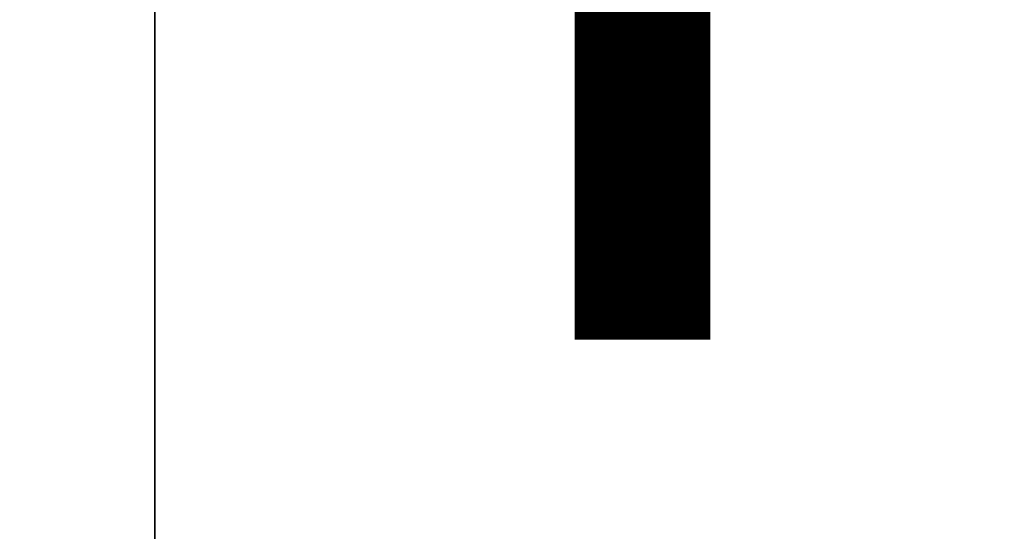
# Model space of a CAD drawing. Units: inches. Extents: x 2083 to 3317, y 1141 to 2115.
# Tile 23 of 256: x 2225.819 to 2234.135, y 1481.434 to 1485.751. Entities that reach past the tile are written whole.
import ezdxf

# ---------------------------------------------------------------- set-up
doc = ezdxf.new("R2010")
doc.units = ezdxf.units.IN
doc.layers.add('A-ANNO-DIMS', color=2, linetype='Continuous', lineweight=18)
doc.layers.add('A-WALL', color=7, linetype='Continuous', lineweight=35)
doc.layers.add('A-WALL-PATT', color=251, linetype='Continuous', lineweight=13, true_color=0x636466)
doc.styles.get("Standard").update_dxf_attribs({"font": 'arial.ttf'})
doc.dimstyles.new('ISO-25', dxfattribs={"dimtxt": 12, "dimasz": 12, "dimexe": 1.25, "dimexo": 0.625, "dimtad": 1, "dimlunit": 3, "dimtxsty": 'Standard', "dimcen": 2.5, "dimadec": 0, "dimazin": 0, "dimtfac": 1, "dimtmove": 0, "dimatfit": 3, "dimfxl": 1, "dimarcsym": 0})

# ---------------------------------------------------------------- blocks, each defined once
blk = doc.blocks.new('*D30')
at = {"layer": 'A-ANNO-DIMS', "color": 0, "lineweight": -2, "transparency": 16777216}
for p, q in [((2240.0179, 1445.2738), (2240.0179, 1448.0455)), ((2254.3293, 1445.2738), (2254.3293, 1448.0455)), ((2228.0179, 1446.7955), (2216.0179, 1446.7955)), ((2240.0179, 1446.7955), (2254.3293, 1446.7955)), ((2266.3293, 1446.7955), (2413.7649, 1446.7955))]:
    blk.add_line(p, q, dxfattribs=at)
at = {"layer": 'A-ANNO-DIMS', "color": 0, "transparency": 16777216}
for points in [[(2228.0179, 1448.7955), (2228.0179, 1444.7955), (2240.0179, 1446.7955)], [(2266.3293, 1448.7955), (2266.3293, 1444.7955), (2254.3293, 1446.7955)]]:
    blk.add_solid(points, dxfattribs=at)
at = {"layer": 'Defpoints', "color": 0, "transparency": 16777216}
for p in [(2254.3293, 1446.7955), (2240.0179, 1444.6488), (2254.3293, 1444.6488)]:
    blk.add_point(p, dxfattribs=at)
at = {"layer": 'A-ANNO-DIMS', "color": 0, "transparency": 16777216, "insert": (2346.0471, 1453.6252), "char_height": 12, "attachment_point": 5}
blk.add_mtext('WC 1\'-2 1/2" TYP.', dxfattribs=at)
blk = doc.blocks.new('*D31')
at = {"layer": 'A-ANNO-DIMS', "color": 0, "lineweight": -2, "transparency": 16777216}
for p, q in [((2237.8711, 1456.6488), (2237.8711, 1541.9152)), ((2239.3929, 1444.6488), (2236.6211, 1444.6488)), ((2237.8711, 1431.5475), (2237.8711, 1444.6488)), ((2239.3929, 1431.5475), (2236.6211, 1431.5475)), ((2237.8711, 1419.5475), (2237.8711, 1407.5475))]:
    blk.add_line(p, q, dxfattribs=at)
at = {"layer": 'A-ANNO-DIMS', "color": 0, "transparency": 16777216}
for points in [[(2235.8711, 1456.6488), (2239.8711, 1456.6488), (2237.8711, 1444.6488)], [(2235.8711, 1419.5475), (2239.8711, 1419.5475), (2237.8711, 1431.5475)]]:
    blk.add_solid(points, dxfattribs=at)
at = {"layer": 'Defpoints', "color": 0, "transparency": 16777216}
for p in [(2237.8711, 1444.6488), (2240.0179, 1444.6488), (2240.0179, 1431.5475)]:
    blk.add_point(p, dxfattribs=at)
at = {"layer": 'A-ANNO-DIMS', "color": 0, "transparency": 16777216, "insert": (2231.2175, 1505.282), "char_height": 12, "attachment_point": 5, "rotation": 90}
blk.add_mtext('1\'-1" TYP.', dxfattribs=at)

msp = doc.modelspace()

# ---------------------------------------------------------------- hatches: boundary and pattern name
at = {"layer": 'A-WALL-PATT'}
h = msp.add_hatch(color=256, dxfattribs=at)
h.dxf.hatch_style = 1
h.paths.add_polyline_path([(3126.9598, 2020.7614), (2748.9598, 2020.7614), (2604.9598, 2020.7614), (2226.9598, 2020.7614), (2226.9598, 1702.7614), (2466.9598, 1702.7614), (2466.9598, 1582.7614), (2418.9598, 1582.7614), (2418.9598, 1477.7614), (2226.9598, 1477.7614), (2226.9598, 1263.2614), (2544.9598, 1263.2614), (2544.9598, 1411.7614), (2604.9598, 1411.7614), (2685.9598, 1411.7614), (2685.9598, 1420.7614), (2604.9598, 1420.7614), (2604.9598, 1573.7614), (2604.9598, 1702.7614), (2604.9598, 2011.7614), (2748.9598, 2011.7614), (2748.9598, 1702.7614), (2862.9598, 1702.7614), (2862.9598, 1621.7614), (2871.9598, 1621.7614), (2871.9598, 1702.7614), (2883.9598, 1702.7614), (2883.9598, 1706.9395, -0.026459), (2883.9598, 1711.7614), (2757.9598, 1711.7614), (2757.9598, 1807.7614), (2787.9598, 1807.7614), (2787.9598, 1812.2614), (2757.9598, 1812.2614), (2757.9598, 2011.7614), (2877.9598, 2011.7614), (2877.9598, 1812.2614), (2847.9598, 1812.2614), (2847.9598, 1807.7614), (2889.8357, 1807.7614), (2889.8357, 1812.2614), (2882.4598, 1812.2614), (2882.4598, 2011.7614), (3117.9598, 2011.7614), (3117.9598, 1812.2614), (2937.8357, 1812.2614), (2937.8357, 1807.7614), (2995.7098, 1807.7614), (2995.7098, 1796.1177), (3000.2098, 1796.1177), (3000.2098, 1807.7614), (3117.9598, 1807.7614), (3117.9598, 1711.7614), (3000.2098, 1711.7614), (3000.2098, 1760.1177), (2998.5727, 1760.1177, -0.020711), (2995.7098, 1760.1177), (2995.7098, 1711.7614), (2931.9598, 1711.7614), (2931.9598, 1702.7614), (3126.9598, 1702.7614)])
h.paths.add_polyline_path([(2471.4598, 2011.7614), (2471.4598, 1810.0114), (2462.7169, 1810.0114), (2462.7169, 1805.5114), (2505.9598, 1805.5114), (2505.9598, 1810.0114), (2475.9598, 1810.0114), (2475.9598, 2011.7614), (2595.9598, 2011.7614), (2595.9598, 1810.0114), (2565.9598, 1810.0114), (2565.9598, 1805.5114), (2595.9598, 1805.5114), (2595.9598, 1711.7614), (2235.9598, 1711.7614), (2235.9598, 1805.5114), (2353.7098, 1805.5114), (2353.7098, 1796.0542), (2358.2098, 1796.0542), (2358.2098, 1805.5114), (2414.7169, 1805.5114), (2414.7169, 1810.0114), (2235.9598, 1810.0114), (2235.9598, 2011.7614)], flags=16)
h.paths.add_polyline_path([(2270.2047, 1994.61), (2270.2047, 1970.61), (2246.2047, 1970.61), (2246.2047, 1994.61)], flags=0)
edge = h.paths.add_edge_path(flags=0)
edge.add_ellipse((2332.0274, 1899.7982), major_axis=(-3.043, 3.043), ratio=0.168252, start_angle=-161.33217, end_angle=-156.30711, ccw=False)
edge.add_ellipse((2333.082, 1898.7435), major_axis=(-1.0546, 1.0546), ratio=0.453532, start_angle=-123.37102, end_angle=-94.15911)
edge = h.paths.add_edge_path(flags=0)
edge.add_ellipse((2332.0274, 1968.8763), major_axis=(3.043, 3.043), ratio=0.168252, start_angle=18.66783, end_angle=23.69289)
edge.add_spline(control_points=[(2332.9256, 1970.6911), (2332.2268, 1970.3361), (2330.8937, 1969.6589), (2328.4131, 1970.9321), (2327.2039, 1967.7487), (2324.7096, 1969.9556), (2322.5328, 1967.0124), (2320.0128, 1971.2958), (2317.6803, 1968.1578), (2316.0405, 1967.102), (2315.4269, 1966.8096)], knot_values=[0, 0, 0, 0, 2.267059, 4.324559, 6.685584, 8.878641, 11.121502, 14.300359, 17.755284, 19.732645, 19.732645, 19.732645, 19.732645], degree=3, periodic=0)
edge.add_ellipse((2332.0274, 1968.8763), major_axis=(3.043, 3.043), ratio=0.168252, start_angle=18.66783, end_angle=23.69289, ccw=False)
edge.add_ellipse((2333.082, 1969.9309), major_axis=(1.0546, 1.0546), ratio=0.453532, start_angle=56.62898, end_angle=85.84089, ccw=False)
edge = h.paths.add_edge_path(flags=0)
edge.add_spline(control_points=[(2296.4283, 1967.9879), (2293.6278, 1965.3363), (2287.7036, 1959.7271), (2299.7439, 1949.9957), (2294.5326, 1935.6685), (2290.5732, 1920.6035), (2293.3941, 1909.9737), (2296.1854, 1904.9665)], knot_values=[0.099185, 0.099185, 0.099185, 0.099185, 0.345301, 0.619822, 0.982653, 1.386093, 1.810555, 1.810555, 1.810555, 1.810555], degree=3, periodic=0)
edge.add_spline(control_points=[(2296.1854, 1904.9665), (2297.3836, 1902.6193), (2298.001, 1901.9493), (2298.553, 1901.4682)], knot_values=[0.006246, 0.006246, 0.006246, 0.006246, 0.055476, 0.055476, 0.055476, 0.055476], degree=3, periodic=0)
edge.add_spline(control_points=[(2298.553, 1901.4682), (2297.2586, 1900.9232), (2295.2253, 1900.2321), (2293.0602, 1900.6142), (2292.1014, 1900.7884), (2292.0896, 1900.7906)], knot_values=[0.312835, 0.312835, 0.312835, 0.312835, 0.40178, 0.474987, 0.475903, 0.475903, 0.475903, 0.475903], degree=3, periodic=0)
edge.add_arc((2292.7936, 1904.6641), 3.937, 215.4209, 259.69818, ccw=False)
edge.add_spline(control_points=[(2289.5853, 1902.3823), (2289.4767, 1902.5351), (2289.3685, 1902.688), (2289.2609, 1902.8412)], knot_values=[0.102872, 0.102872, 0.102872, 0.102872, 0.116896, 0.116896, 0.116896, 0.116896], degree=3, periodic=0)
edge.add_spline(control_points=[(2289.2609, 1902.8412), (2288.6866, 1902.5502), (2287.64, 1902.0199), (2285.8813, 1901.874), (2283.853, 1901.5044), (2281.72, 1899.7105), (2278.467, 1899.4929), (2276.1571, 1901.8832), (2272.259, 1899.8041), (2267.7776, 1901.8432), (2262.2439, 1900.184), (2257.4149, 1901.7821), (2254.3184, 1900.7261), (2253.1783, 1900.3373)], knot_values=[0, 0, 0, 0, 1.907977, 3.477176, 5.261074, 7.972851, 11.680248, 13.717921, 16.939592, 22.789562, 27.502503, 33.595215, 37.145618, 37.145618, 37.145618, 37.145618], degree=3, periodic=0)
edge.add_line((2253.1783, 1900.3373), (2250.2442, 1902.8412))
edge.add_line((2250.2442, 1902.8412), (2250.2442, 1965.8333))
edge.add_line((2250.2442, 1965.8333), (2253.1783, 1968.3371))
edge.add_spline(control_points=[(2253.1783, 1968.3371), (2254.3184, 1967.9483), (2257.4149, 1966.8924), (2262.2439, 1968.4904), (2267.7776, 1966.8313), (2271.5267, 1968.5372), (2273.8759, 1967.8283), (2274.2067, 1967.7276)], knot_values=[0, 0, 0, 0, 0.09018, 0.244935, 0.364644, 0.513233, 0.537855, 0.537855, 0.537855, 0.537855], degree=3, periodic=0)
edge.add_arc((2274.3529, 1963.7933), 3.937, 72.05113, 92.12795, ccw=False)
edge.add_arc((2281.2969, 1985.23), 18.5963, 252.05113, 288.56572)
edge.add_arc((2292.3167, 1956.0289), 12.6461, 71.02679, 113.77822, ccw=False)
edge = h.paths.add_edge_path(flags=0)
edge.add_spline(control_points=[(2274.8994, 1951.8562), (2275.0662, 1951.6166), (2275.2327, 1951.3766), (2275.398, 1951.1359)], knot_values=[1.409916, 1.409916, 1.409916, 1.409916, 1.43159, 1.43159, 1.43159, 1.43159], degree=3, periodic=0)
edge.add_spline(control_points=[(2275.398, 1951.1359), (2275.7921, 1950.5619), (2276.1792, 1949.9838), (2276.5455, 1949.3971)], knot_values=[1.358238, 1.358238, 1.358238, 1.358238, 1.409916, 1.409916, 1.409916, 1.409916], degree=3, periodic=0)
edge.add_line((2276.5455, 1949.3971), (2277.4373, 1947.8622))
edge.add_spline(control_points=[(2277.4373, 1947.8622), (2276.3038, 1945.6731), (2274.6397, 1942.4269), (2274.6316, 1938.0939), (2272.7991, 1930.8515), (2274.3564, 1943.897), (2275.9477, 1947.9234), (2276.5455, 1949.3971)], knot_values=[0.005632, 0.005632, 0.005632, 0.005632, 0.186014, 0.266002, 0.357087, 0.59639, 0.739732, 0.739732, 0.739732, 0.739732], degree=3, periodic=0)
edge.add_spline(control_points=[(2276.5455, 1949.3971), (2276.1792, 1949.9838), (2275.7921, 1950.5619), (2275.398, 1951.1359)], knot_values=[1.358238, 1.358238, 1.358238, 1.358238, 1.409916, 1.409916, 1.409916, 1.409916], degree=3, periodic=0)
edge.add_spline(control_points=[(2275.398, 1951.1359), (2274.9425, 1950.0805), (2274.2078, 1948.0253), (2273.9346, 1944.8515), (2272.4685, 1937.6275), (2273.4662, 1945.6965), (2274.7006, 1951.0595), (2274.8994, 1951.8562)], knot_values=[0.104364, 0.104364, 0.104364, 0.104364, 0.189636, 0.269624, 0.36071, 0.600013, 0.644622, 0.644622, 0.644622, 0.644622], degree=3, periodic=0)
h.paths.add_polyline_path([(2269.1675, 1963.1276, -0.357527), (2268.1706, 1960.9764, -0.092561), (2268.1706, 1939.4363, -0.357527), (2269.1675, 1937.2851, -0.357527), (2267.0163, 1938.282, -0.164785), (2254.6856, 1938.282, -0.357527), (2252.5344, 1937.2851, -0.357527), (2253.5313, 1939.4363, -0.092561), (2253.5313, 1960.9764, -0.357527), (2252.5344, 1963.1276, -0.357527), (2254.6856, 1962.1307, -0.164785), (2267.0163, 1962.1307, -0.357527)], flags=0)
h.paths.add_polyline_path([(2248.8741, 1967.8018), (2248.8741, 1957.0277), (2249.4578, 1957.0277), (2249.4578, 1911.6468), (2248.8741, 1911.6468), (2248.8741, 1900.8727), (2246.5119, 1900.8727, 0.197327), (2244.1497, 1902.4569), (2244.1497, 1966.2176, 0.197327), (2246.5119, 1967.8018)], flags=0)
h.paths.add_polyline_path([(2269.1675, 1931.3893, -0.357527), (2268.1706, 1929.2381, -0.092561), (2268.1706, 1907.6981, -0.357527), (2269.1675, 1905.5469, -0.357527), (2267.0163, 1906.5438, -0.164785), (2254.6856, 1906.5438, -0.357527), (2252.5344, 1905.5469, -0.357527), (2253.5313, 1907.6981, -0.092561), (2253.5313, 1929.2381, -0.357527), (2252.5344, 1931.3893, -0.357527), (2254.6856, 1930.3925, -0.164785), (2267.0163, 1930.3925, -0.357527)], flags=0)
edge = h.paths.add_edge_path(flags=0)
edge.add_spline(control_points=[(2276.1969, 1906.7237), (2276.1681, 1909.0289), (2276.114, 1913.3719), (2270.5984, 1924.925), (2273.9052, 1919.0128), (2275.9217, 1916.2621), (2275.4746, 1912.4021), (2277.2579, 1910.3806), (2276.696, 1908.225), (2276.6462, 1906.813), (2276.6178, 1906.0084)], knot_values=[0, 0, 0, 0, 8.61026, 16.221274, 18.843057, 23.804898, 27.440828, 29.356102, 31.203478, 33.650687, 33.650687, 33.650687, 33.650687], degree=3, periodic=0)
edge.add_spline(control_points=[(2276.6178, 1906.0084), (2276.6233, 1905.6241), (2276.4977, 1904.6287), (2275.4418, 1903.8547), (2274.9373, 1903.0804), (2274.8591, 1902.8412)], knot_values=[0.156488, 0.156488, 0.156488, 0.156488, 0.184398, 0.231376, 0.250598, 0.250598, 0.250598, 0.250598], degree=3, periodic=0)
edge.add_line((2274.8591, 1902.8412), (2276.506, 1902.8412))
edge.add_spline(control_points=[(2276.506, 1902.8412), (2276.7883, 1903.0849), (2277.6651, 1904.1252), (2278.2495, 1904.3407), (2277.6539, 1908.5274), (2278.1557, 1906.2278), (2278.1005, 1905.2859), (2278.8467, 1904.069), (2277.8568, 1903.4149), (2277.8742, 1902.991), (2277.9036, 1902.8412)], knot_values=[0.059574, 0.059574, 0.059574, 0.059574, 0.080753, 0.103741, 0.16972, 0.176036, 0.207137, 0.240474, 0.262341, 0.27366, 0.27366, 0.27366, 0.27366], degree=3, periodic=0)
edge.add_line((2277.9036, 1902.8412), (2280.0298, 1902.8412))
edge.add_spline(control_points=[(2280.0298, 1902.8412), (2279.8882, 1903.0884), (2279.4993, 1903.9816), (2280.1523, 1905.9393), (2278.1036, 1909.6578), (2279.7624, 1907.1853), (2280.3279, 1904.8749), (2280.4851, 1903.4896), (2281.4633, 1903.2494), (2281.7583, 1902.9365), (2281.834, 1902.8412)], knot_values=[0.013856, 0.013856, 0.013856, 0.013856, 0.034874, 0.088867, 0.107879, 0.126738, 0.158714, 0.193757, 0.217487, 0.226722, 0.226722, 0.226722, 0.226722], degree=3, periodic=0)
edge.add_spline(control_points=[(2281.834, 1902.8412), (2281.7875, 1902.8267), (2281.647, 1902.783), (2281.3955, 1902.8595), (2281.0881, 1902.9852), (2280.7207, 1903.0609), (2280.3335, 1903.0257), (2280.1248, 1902.8989), (2280.0298, 1902.8412)], knot_values=[0, 0, 0, 0, 0.14413, 0.435517, 0.749276, 1.153046, 1.548371, 1.878348, 1.878348, 1.878348, 1.878348], degree=3, periodic=0)
edge.add_line((2280.0298, 1902.8412), (2277.9036, 1902.8412))
edge.add_spline(control_points=[(2277.9036, 1902.8412), (2277.8929, 1902.7959), (2277.8654, 1902.6796), (2277.6075, 1902.6875), (2277.2741, 1902.8007), (2276.8379, 1902.6198), (2276.5838, 1902.7893), (2276.506, 1902.8412)], knot_values=[0, 0, 0, 0, 0.127189, 0.326199, 0.628009, 1.24357, 1.515331, 1.515331, 1.515331, 1.515331], degree=3, periodic=0)
edge.add_line((2276.506, 1902.8412), (2274.8591, 1902.8412))
edge.add_spline(control_points=[(2274.8591, 1902.8412), (2274.8144, 1902.8986), (2274.7251, 1903.0134), (2274.4935, 1903.119), (2274.2443, 1902.9605), (2273.9371, 1903.1849), (2273.614, 1902.9831), (2273.4083, 1902.883), (2273.3223, 1902.8412)], knot_values=[0, 0, 0, 0, 0.21843, 0.436957, 0.687977, 0.990379, 1.398396, 1.69185, 1.69185, 1.69185, 1.69185], degree=3, periodic=0)
edge.add_spline(control_points=[(2273.3223, 1902.8412), (2273.6167, 1903.4457), (2274.274, 1904.5383), (2276.0272, 1904.5737), (2276.207, 1906.5836), (2276.1969, 1906.7237)], knot_values=[0.012227, 0.012227, 0.012227, 0.012227, 0.059472, 0.106218, 0.134458, 0.134458, 0.134458, 0.134458], degree=3, periodic=0)
h.paths.add_polyline_path([(2270.7761, 1897.7898), (2270.7761, 1873.7898), (2246.7761, 1873.7898), (2246.7761, 1897.7898)], flags=0)
h.paths.add_polyline_path([(2353.7098, 1760.0051), (2353.7098, 1760.0542), (2358.2098, 1760.0542, -0.033729)], flags=0)
h.paths.add_polyline_path([(2321.8191, 1737.5292), (2341.9953, 1737.5292, -0.414214), (2343.2033, 1736.3212), (2343.2033, 1721.0206, -0.414214), (2341.9953, 1719.8127), (2321.8191, 1719.8127, -0.414214), (2320.6112, 1721.0206), (2320.6112, 1736.3212, -0.414214)], flags=0)
h.paths.add_polyline_path([(2324.235, 1736.3212), (2339.5794, 1736.3212, -0.414214), (2341.9953, 1733.9053), (2341.9953, 1725.4497, -0.414214), (2339.5794, 1723.0338), (2333.6806, 1723.0338), (2333.8453, 1722.0455, -0.870646), (2335.4254, 1721.8259, -0.767327), (2333.9227, 1721.4232), (2331.291, 1721.4232, -0.767327), (2329.7883, 1721.8259, -0.870646), (2331.3684, 1722.0455), (2331.5331, 1723.0338), (2324.235, 1723.0338, -0.414214), (2321.8191, 1725.4497), (2321.8191, 1733.9053, -0.414214)], flags=0)
h.paths.add_polyline_path([(2570.4838, 1928.6154), (2589.6838, 1928.6154), (2590.1688, 1928.6154), (2590.1688, 1904.9934), (2570.4838, 1904.9934)], flags=0)
h.paths.add_polyline_path([(2574.4473, 1927.2638, -1), (2572.8288, 1927.2638, -1)], flags=0)
h.paths.add_polyline_path([(2573.0899, 1926.9409), (2573.925, 1927.776), (2574.1477, 1927.5533), (2573.3126, 1926.7182)], flags=0)
h.paths.add_polyline_path([(2578.7791, 1919.7296, -1), (2571.5917, 1919.7296, -1)], flags=0)
h.paths.add_polyline_path([(2578.3854, 1919.7296, -1), (2571.9854, 1919.7296, -1)], flags=0)
h.paths.add_polyline_path([(2331.5958, 1729.4762, -1), (2333.618, 1729.4762, -1)], flags=0)
h.paths.add_polyline_path([(2578.0342, 1927.2638, -1), (2576.4157, 1927.2638, -1)], flags=0)
h.paths.add_polyline_path([(2576.6889, 1927.5311), (2576.9116, 1927.7538), (2577.7467, 1926.9186), (2577.524, 1926.6959)], flags=0)
h.paths.add_polyline_path([(2578.1391, 1909.8595, -1), (2572.2317, 1909.8595, -1)], flags=0)
h.paths.add_polyline_path([(2577.7454, 1909.8595, -1), (2572.6254, 1909.8595, -1)], flags=0)
h.paths.add_polyline_path([(2583.7977, 1927.2638, -1), (2582.1792, 1927.2638, -1)], flags=0)
h.paths.add_polyline_path([(2582.7186, 1927.7538), (2583.5538, 1926.9186), (2583.3311, 1926.6959), (2582.4959, 1927.5311)], flags=0)
h.paths.add_polyline_path([(2582.4959, 1927.5311), (2582.7186, 1927.7538), (2583.5538, 1926.9186), (2583.3311, 1926.6959)], flags=0)
h.paths.add_polyline_path([(2587.7391, 1920.5296, -1), (2581.8317, 1920.5296, -1)], flags=0)
h.paths.add_polyline_path([(2587.3454, 1920.5296, -1), (2582.2254, 1920.5296, -1)], flags=0)
h.paths.add_polyline_path([(2587.3846, 1927.2638, -1), (2585.7661, 1927.2638, -1)], flags=0)
h.paths.add_polyline_path([(2586.082, 1926.9802), (2586.9172, 1927.8154), (2587.1399, 1927.5927), (2586.3047, 1926.7575)], flags=0)
h.paths.add_polyline_path([(2588.3791, 1910.6595, -1), (2581.1917, 1910.6595, -1)], flags=0)
h.paths.add_polyline_path([(2587.9854, 1910.6595, -1), (2581.5854, 1910.6595, -1)], flags=0)
h.paths.add_polyline_path([(2417.1677, 1729.4779), (2437.3439, 1729.4779, -0.414214), (2438.5519, 1728.2699), (2438.5519, 1712.9693, -0.414214), (2437.3439, 1711.7614), (2417.1677, 1711.7614, -0.414214), (2415.9598, 1712.9693), (2415.9598, 1728.2699, -0.414214)], flags=0)
h.paths.add_polyline_path([(2419.5836, 1728.2699), (2434.928, 1728.2699, -0.414214), (2437.3439, 1725.8541), (2437.3439, 1717.3984, -0.414214), (2434.928, 1714.9825), (2429.0292, 1714.9825), (2429.1939, 1713.9942, -0.870646), (2430.774, 1713.7746, -0.767327), (2429.2713, 1713.372), (2426.6396, 1713.372, -0.767327), (2425.1369, 1713.7746, -0.870646), (2426.717, 1713.9942), (2426.8817, 1714.9825), (2419.5836, 1714.9825, -0.414214), (2417.1677, 1717.3984), (2417.1677, 1725.8541, -0.414214)], flags=0)
h.paths.add_polyline_path([(2419.5836, 1728.2699), (2434.928, 1728.2699, -0.414214), (2437.3439, 1725.8541), (2437.3439, 1717.3984, -0.414214), (2434.928, 1714.9825), (2429.0292, 1714.9825), (2428.3581, 1719.009), (2427.5528, 1719.009), (2426.8817, 1714.9825), (2419.5836, 1714.9825, -0.414214), (2417.1677, 1717.3984), (2417.1677, 1725.8541, -0.414214)], flags=0)
h.paths.add_polyline_path([(2426.9444, 1721.4249, -1), (2428.9666, 1721.4249, -1)], flags=0)
h.paths.add_polyline_path([(2475.9598, 1702.7614), (2595.9598, 1702.7614), (2595.9598, 1582.7614), (2475.9598, 1582.7614)], flags=16)
h.paths.add_polyline_path([(2427.9598, 1573.7614), (2595.9598, 1573.7614), (2595.9598, 1468.7614), (2595.9598, 1420.7614), (2384.4598, 1420.7614), (2384.4598, 1468.7614), (2427.9598, 1468.7614)], flags=16)
h.paths.add_polyline_path([(2379.9598, 1468.7614), (2379.9598, 1420.7614), (2235.9598, 1420.7614), (2235.9598, 1468.7614)], flags=16)
h.paths.add_polyline_path([(2317.816, 1466.6958), (2337.9922, 1466.6958, -0.414214), (2339.2002, 1465.4878), (2339.2002, 1450.1872, -0.414214), (2337.9922, 1448.9792), (2317.816, 1448.9792, -0.414214), (2316.6081, 1450.1872), (2316.6081, 1465.4878, -0.414214)], flags=0)
h.paths.add_polyline_path([(2320.2319, 1465.4878), (2335.5763, 1465.4878, -0.414214), (2337.9922, 1463.0719), (2337.9922, 1454.6163, -0.414214), (2335.5763, 1452.2004), (2329.6775, 1452.2004), (2329.8422, 1451.212, -0.870646), (2331.4223, 1450.9925, -0.767327), (2329.9196, 1450.5898), (2327.2879, 1450.5898, -0.767327), (2325.7852, 1450.9925, -0.870646), (2327.3653, 1451.212), (2327.53, 1452.2004), (2320.2319, 1452.2004, -0.414214), (2317.816, 1454.6163), (2317.816, 1463.0719, -0.414214)], flags=0)
h.paths.add_polyline_path([(2320.2319, 1465.4878), (2335.5763, 1465.4878, -0.414214), (2337.9922, 1463.0719), (2337.9922, 1454.6163, -0.414214), (2335.5763, 1452.2004), (2329.6775, 1452.2004), (2329.0064, 1456.2269), (2328.2011, 1456.2269), (2327.53, 1452.2004), (2320.2319, 1452.2004, -0.414214), (2317.816, 1454.6163), (2317.816, 1463.0719, -0.414214)], flags=0)
h.paths.add_polyline_path([(2327.5926, 1458.6428, -1), (2329.6148, 1458.6428, -1)], flags=0)
h.paths.add_polyline_path([(2244.4117, 1433.3405), (2241.9209, 1433.3405, -0.414214), (2240.0179, 1435.2435), (2240.0179, 1440.9528, -0.414211), (2241.9209, 1442.8559), (2244.4117, 1442.8559, -1.976472)], flags=0)
h.paths.add_polyline_path([(2245.3569, 1434.3975, -0.414214), (2245.3569, 1441.7988, -2.144098)], flags=0)
h.paths.add_polyline_path([(2535.9598, 1416.2614), (2535.9598, 1272.2614), (2235.9598, 1272.2614), (2235.9598, 1416.2614)], flags=16)
h.paths.add_polyline_path([(2260.1196, 1384.2928), (2260.1196, 1362.0386), (2237.8654, 1362.0386), (2237.8654, 1384.2928)], flags=0)
edge = h.paths.add_edge_path(flags=0)
edge.add_line((2318.2518, 1362.0933), (2318.1458, 1362.001))
edge.add_ellipse((2317.4451, 1360.431), major_axis=(2.8216, 2.8216), ratio=0.168252, start_angle=18.66783, end_angle=20.94813, ccw=False)
edge.add_ellipse((2318.423, 1361.409), major_axis=(0.9779, 0.9779), ratio=0.453532, start_angle=56.62898, end_angle=70.2262, ccw=False)
edge = h.paths.add_edge_path(flags=0)
edge.add_line((2319.1074, 1295.5711), (2319.015, 1295.6771))
edge.add_ellipse((2317.4451, 1296.3778), major_axis=(-2.8216, 2.8216), ratio=0.168252, start_angle=-161.33217, end_angle=-159.05187, ccw=False)
edge.add_ellipse((2318.423, 1295.3999), major_axis=(-0.9779, 0.9779), ratio=0.453532, start_angle=-123.37102, end_angle=-109.7738)
edge = h.paths.add_edge_path(flags=0)
edge.add_spline(control_points=[(2284.2103, 1301.1702), (2284.5807, 1300.4447), (2284.8912, 1299.892), (2285.1596, 1299.461)], knot_values=[0.039066, 0.039066, 0.039066, 0.039066, 0.055476, 0.055476, 0.055476, 0.055476], degree=3, periodic=0)
edge.add_line((2285.1596, 1299.461), (2284.2103, 1301.1702))
edge = h.paths.add_edge_path(flags=0)
edge.add_line((2280.4125, 1297.298), (2283.37, 1297.0361))
edge.add_line((2283.37, 1297.0361), (2286.4057, 1297.9263))
edge.add_spline(control_points=[(2286.4057, 1297.9263), (2285.3055, 1297.4631), (2284.3448, 1297.1292), (2283.37, 1297.0361)], knot_values=[0.394369, 0.394369, 0.394369, 0.394369, 0.475903, 0.475903, 0.475903, 0.475903], degree=3, periodic=0)
edge.add_spline(control_points=[(2283.37, 1297.0361), (2283.2814, 1297.0277), (2282.3163, 1296.9573), (2281.3125, 1297.1345), (2280.4234, 1297.296), (2280.4125, 1297.298)], knot_values=[0.312835, 0.312835, 0.312835, 0.312835, 0.320246, 0.393453, 0.394369, 0.394369, 0.394369, 0.394369], degree=3, periodic=0)
edge = h.paths.add_edge_path(flags=0)
edge.add_line((2284.4356, 1359.6073), (2280.4463, 1355.328))
edge.add_line((2280.4463, 1355.328), (2279.58, 1351.0178))
edge.add_line((2279.58, 1351.0178), (2282.413, 1346.5804))
edge.add_spline(control_points=[(2282.413, 1346.5804), (2283.1533, 1345.5892), (2284.2529, 1344.0289), (2284.801, 1342.3872), (2284.9352, 1341.8055)], knot_values=[1.240098, 1.240098, 1.240098, 1.240098, 1.332892, 1.382712, 1.382712, 1.382712, 1.382712], degree=3, periodic=0)
edge.add_spline(control_points=[(2284.9352, 1341.8055), (2285.3191, 1340.1406), (2285.233, 1338.4092), (2284.9099, 1336.6541)], knot_values=[1.097484, 1.097484, 1.097484, 1.097484, 1.240098, 1.240098, 1.240098, 1.240098], degree=3, periodic=0)
edge.add_spline(control_points=[(2284.9099, 1336.6541), (2284.5868, 1334.899), (2284.0267, 1333.1203), (2283.4626, 1331.3606)], knot_values=[0.95487, 0.95487, 0.95487, 0.95487, 1.097484, 1.097484, 1.097484, 1.097484], degree=3, periodic=0)
edge.add_line((2283.4626, 1331.3606), (2281.8904, 1326.1534))
edge.add_line((2281.8904, 1326.1534), (2280.7563, 1321.0561))
edge.add_line((2280.7563, 1321.0561), (2280.2992, 1316.002))
edge.add_line((2280.2992, 1316.002), (2280.7159, 1310.9501))
edge.add_line((2280.7159, 1310.9501), (2282.0281, 1305.9721))
edge.add_line((2282.0281, 1305.9721), (2284.2103, 1301.1702))
edge.add_spline(control_points=[(2284.2103, 1301.1702), (2283.3407, 1302.7302), (2282.6119, 1304.3365), (2282.0281, 1305.9721)], knot_values=[0.099185, 0.099185, 0.099185, 0.099185, 0.241799, 0.241799, 0.241799, 0.241799], degree=3, periodic=0)
edge.add_spline(control_points=[(2282.0281, 1305.9721), (2281.4443, 1307.6078), (2281.0055, 1309.2728), (2280.7159, 1310.9501)], knot_values=[0.241799, 0.241799, 0.241799, 0.241799, 0.384413, 0.384413, 0.384413, 0.384413], degree=3, periodic=0)
edge.add_spline(control_points=[(2280.7159, 1310.9501), (2280.4332, 1312.5876), (2280.2894, 1314.277), (2280.2989, 1315.962), (2280.2992, 1316.002)], knot_values=[0.384413, 0.384413, 0.384413, 0.384413, 0.523647, 0.527028, 0.527028, 0.527028, 0.527028], degree=3, periodic=0)
edge.add_spline(control_points=[(2280.2992, 1316.002), (2280.3123, 1317.687), (2280.4779, 1319.3679), (2280.7563, 1321.0561)], knot_values=[0.527028, 0.527028, 0.527028, 0.527028, 0.669642, 0.669642, 0.669642, 0.669642], degree=3, periodic=0)
edge.add_spline(control_points=[(2280.7563, 1321.0561), (2281.0346, 1322.7443), (2281.4259, 1324.4396), (2281.8904, 1326.1534)], knot_values=[0.669642, 0.669642, 0.669642, 0.669642, 0.812256, 0.812256, 0.812256, 0.812256], degree=3, periodic=0)
edge.add_spline(control_points=[(2281.8904, 1326.1534), (2282.2644, 1327.5333), (2282.7879, 1329.2618), (2283.3528, 1331.0178), (2283.4626, 1331.3606)], knot_values=[0.812256, 0.812256, 0.812256, 0.812256, 0.927087, 0.95487, 0.95487, 0.95487, 0.95487], degree=3, periodic=0)
edge.add_line((2283.4626, 1331.3606), (2284.9099, 1336.6541))
edge.add_line((2284.9099, 1336.6541), (2284.9352, 1341.8055))
edge.add_line((2284.9352, 1341.8055), (2282.413, 1346.5804))
edge.add_spline(control_points=[(2282.413, 1346.5804), (2281.2751, 1348.1038), (2280.0784, 1349.5703), (2279.58, 1351.0178)], knot_values=[1.382712, 1.382712, 1.382712, 1.382712, 1.525326, 1.525326, 1.525326, 1.525326], degree=3, periodic=0)
edge.add_spline(control_points=[(2279.58, 1351.0178), (2279.4433, 1351.4147), (2279.1363, 1352.8569), (2279.7352, 1354.2904), (2280.4463, 1355.328)], knot_values=[1.525326, 1.525326, 1.525326, 1.525326, 1.564439, 1.667941, 1.667941, 1.667941, 1.667941], degree=3, periodic=0)
edge.add_spline(control_points=[(2280.4463, 1355.328), (2281.4261, 1356.7578), (2282.9308, 1358.1826), (2284.4356, 1359.6073)], knot_values=[1.667941, 1.667941, 1.667941, 1.667941, 1.810555, 1.810555, 1.810555, 1.810555], degree=3, periodic=0)
edge.add_arc((2280.6231, 1348.5182), 11.7262, 71.02679, 113.77822)
edge.add_arc((2270.4049, 1375.5952), 17.2436, 252.05113, 288.56572, ccw=False)
edge.add_arc((2263.966, 1355.7178), 3.6506, 72.05113, 92.12795)
edge.add_arc((2263.966, 1355.7178), 3.6506, 92.12795, 177.98513)
edge.add_spline(control_points=[(2260.3176, 1355.8462), (2260.2604, 1354.2207), (2260.5513, 1350.1865), (2262.9993, 1346.7663), (2264.4727, 1344.649)], knot_values=[1.43159, 1.43159, 1.43159, 1.43159, 1.564144, 1.770695, 1.770695, 1.770695, 1.770695], degree=3, periodic=0)
edge.add_line((2264.4727, 1344.649), (2264.9356, 1343.9825))
edge.add_spline(control_points=[(2263.801, 1340.2481), (2263.8432, 1340.5141), (2264.0672, 1341.7565), (2264.5127, 1343.0025), (2264.935, 1343.9811)], knot_values=[0.53657, 0.53657, 0.53657, 0.53657, 0.559349, 0.644622, 0.644622, 0.644622, 0.644622], degree=3, periodic=0)
edge.add_spline(control_points=[(2264.935, 1343.9811), (2265.1178, 1343.715), (2265.2989, 1343.4479), (2265.4768, 1343.1794)], knot_values=[1.384077, 1.384077, 1.384077, 1.384077, 1.409916, 1.409916, 1.409916, 1.409916], degree=3, periodic=0)
edge.add_spline(control_points=[(2265.4768, 1343.1794), (2265.6546, 1342.9108), (2265.8293, 1342.6408), (2265.9991, 1342.3688)], knot_values=[1.358238, 1.358238, 1.358238, 1.358238, 1.384077, 1.384077, 1.384077, 1.384077], degree=3, periodic=0)
edge.add_line((2265.9991, 1342.3688), (2266.826, 1340.9455))
edge.add_spline(control_points=[(2266.826, 1340.9455), (2268.8944, 1337.0897), (2271.3982, 1325.843), (2270.5162, 1310.5686), (2275.9194, 1301.8606), (2277.7895, 1299.1994)], knot_values=[0.116896, 0.116896, 0.116896, 0.116896, 0.472987, 1.050969, 1.313793, 1.313793, 1.313793, 1.313793], degree=3, periodic=0)
edge.add_spline(control_points=[(2277.7895, 1299.1994), (2277.8394, 1299.1285), (2277.8894, 1299.0575), (2277.9396, 1298.9866)], knot_values=[0.109884, 0.109884, 0.109884, 0.109884, 0.116896, 0.116896, 0.116896, 0.116896], degree=3, periodic=0)
edge.add_line((2277.9396, 1298.9866), (2277.7888, 1299.1991))
edge.add_spline(control_points=[(2277.7888, 1299.1991), (2277.2566, 1298.9294), (2276.2864, 1298.4379), (2275.0394, 1298.3344), (2274.3833, 1298.2389), (2274.2153, 1298.2093)], knot_values=[33.12187, 33.12187, 33.12187, 33.12187, 35.029056, 36.598255, 37.144827, 37.144827, 37.144827, 37.144827], degree=3, periodic=0)
edge.add_line((2274.2153, 1298.2093), (2273.0731, 1297.893))
edge.add_spline(control_points=[(2273.0731, 1297.893), (2272.3229, 1297.5798), (2271.0392, 1296.5105), (2269.2484, 1296.2261), (2268.4231, 1296.3747)], knot_values=[26.532584, 26.532584, 26.532584, 26.532584, 29.198919, 31.839101, 31.839101, 31.839101, 31.839101], degree=3, periodic=0)
edge.add_line((2268.4231, 1296.3747), (2263.8785, 1297.4575))
edge.add_spline(control_points=[(2263.8785, 1297.4575), (2263.5561, 1297.3594), (2261.8603, 1296.8387), (2260.2388, 1297.2824), (2258.9335, 1297.5165)], knot_values=[15.919551, 15.919551, 15.919551, 15.919551, 16.939592, 21.226067, 21.226067, 21.226067, 21.226067], degree=3, periodic=0)
edge.add_line((2258.9335, 1297.5165), (2254.0552, 1297.329))
edge.add_spline(control_points=[(2254.0552, 1297.329), (2253.7555, 1297.2958), (2252.1137, 1297.1652), (2250.4619, 1297.5442), (2249.1297, 1297.6679)], knot_values=[5.306517, 5.306517, 5.306517, 5.306517, 6.276435, 10.613034, 10.613034, 10.613034, 10.613034], degree=3, periodic=0)
edge.add_line((2249.1297, 1297.6679), (2244.3316, 1296.8778))
edge.add_line((2244.3316, 1296.8778), (2241.611, 1299.1994))
edge.add_line((2241.611, 1299.1994), (2241.611, 1357.6094))
edge.add_line((2241.611, 1357.6094), (2244.3316, 1359.9311))
edge.add_line((2244.3316, 1359.9311), (2252.7288, 1359.5427))
edge.add_spline(control_points=[(2252.7288, 1359.5427), (2252.8709, 1359.5464), (2253.3057, 1359.5482), (2253.7398, 1359.5143), (2254.0317, 1359.4824)], knot_values=[0.233291, 0.233291, 0.233291, 0.233291, 0.244935, 0.268927, 0.268927, 0.268927, 0.268927], degree=3, periodic=0)
edge.add_line((2254.0317, 1359.4824), (2259.5872, 1359.4164))
edge.add_spline(control_points=[(2259.5872, 1359.4164), (2260.6771, 1359.6285), (2262.0732, 1359.897), (2263.5237, 1359.4593), (2263.8304, 1359.366)], knot_values=[0.422516, 0.422516, 0.422516, 0.422516, 0.513233, 0.537855, 0.537855, 0.537855, 0.537855], degree=3, periodic=0)
edge.add_arc((2263.966, 1355.7178), 3.6506, 72.05113, 92.12795, ccw=False)
edge.add_arc((2270.4049, 1375.5952), 17.2436, 252.05113, 288.56572)
edge.add_arc((2280.6231, 1348.5182), 11.7262, 71.02679, 113.77822, ccw=False)
h.paths.add_polyline_path([(2240.3405, 1359.4347), (2240.3405, 1349.4444), (2240.8818, 1349.4444), (2240.8818, 1307.3645), (2240.3405, 1307.3645), (2240.3405, 1297.3741), (2238.1502, 1297.3741, 0.197327), (2235.9598, 1298.8431), (2235.9598, 1357.9657, 0.197327), (2238.1502, 1359.4347)], flags=0)
h.paths.add_polyline_path([(2259.1578, 1355.1005, -0.357527), (2258.2334, 1353.1058, -0.092561), (2258.2334, 1333.1326, -0.357527), (2259.1578, 1331.1379, -0.357527), (2257.1631, 1332.0622, -0.164785), (2245.7293, 1332.0622, -0.357527), (2243.7346, 1331.1379, -0.357527), (2244.6589, 1333.1326, -0.092561), (2244.6589, 1353.1058, -0.357527), (2243.7346, 1355.1005, -0.357527), (2245.7293, 1354.1761, -0.164785), (2257.1631, 1354.1761, -0.357527)], flags=0)
edge = h.paths.add_edge_path(flags=0)
edge.add_line((2265.9991, 1342.3688), (2266.826, 1340.9455))
edge.add_line((2266.826, 1340.9455), (2265.3076, 1337.8141))
edge.add_line((2265.3076, 1337.8141), (2264.3582, 1334.6529))
edge.add_line((2264.3582, 1334.6529), (2264.262, 1333.7997))
edge.add_spline(control_points=[(2264.262, 1333.7997), (2264.2084, 1333.1871), (2264.1621, 1332.3655), (2264.0071, 1331.4139), (2263.969, 1331.2018)], knot_values=[0.464444, 0.464444, 0.464444, 0.464444, 0.516691, 0.531608, 0.531608, 0.531608, 0.531608], degree=3, periodic=0)
edge.add_spline(control_points=[(2263.969, 1331.2018), (2263.7745, 1330.1189), (2263.4244, 1328.7908), (2263.2574, 1328.5307), (2263.234, 1328.5146)], knot_values=[0.372682, 0.372682, 0.372682, 0.372682, 0.44885, 0.464444, 0.464444, 0.464444, 0.464444], degree=3, periodic=0)
edge.add_spline(control_points=[(2263.234, 1328.5146), (2263.0964, 1328.4202), (2263.1312, 1329.3015), (2263.275, 1330.6157)], knot_values=[0.280919, 0.280919, 0.280919, 0.280919, 0.372682, 0.372682, 0.372682, 0.372682], degree=3, periodic=0)
edge.add_spline(control_points=[(2263.275, 1330.6157), (2263.4187, 1331.93), (2263.6715, 1333.6773), (2263.9699, 1335.315)], knot_values=[0.189157, 0.189157, 0.189157, 0.189157, 0.280919, 0.280919, 0.280919, 0.280919], degree=3, periodic=0)
edge.add_spline(control_points=[(2263.9699, 1335.315), (2264.1005, 1336.0322), (2264.4188, 1337.6219), (2264.7548, 1338.8644), (2264.9474, 1339.4911)], knot_values=[0.097394, 0.097394, 0.097394, 0.097394, 0.137578, 0.189157, 0.189157, 0.189157, 0.189157], degree=3, periodic=0)
edge.add_spline(control_points=[(2264.9474, 1339.4911), (2265.29, 1340.6061), (2265.6442, 1341.494), (2265.9991, 1342.3688)], knot_values=[0.005632, 0.005632, 0.005632, 0.005632, 0.097394, 0.097394, 0.097394, 0.097394], degree=3, periodic=0)
h.paths.add_polyline_path([(2259.1578, 1325.671, -0.357527), (2258.2334, 1323.6763, -0.092561), (2258.2334, 1303.7031, -0.357527), (2259.1578, 1301.7084, -0.357527), (2257.1631, 1302.6327, -0.164785), (2245.7293, 1302.6327, -0.357527), (2243.7346, 1301.7084, -0.357527), (2244.6589, 1303.7031, -0.092561), (2244.6589, 1323.6763, -0.357527), (2243.7346, 1325.671, -0.357527), (2245.7293, 1324.7466, -0.164785), (2257.1631, 1324.7466, -0.357527)], flags=0)
edge = h.paths.add_edge_path(flags=0)
edge.add_spline(control_points=[(2261.7089, 1317.3114), (2261.6795, 1317.4176), (2261.7619, 1317.3885), (2262.4907, 1316.0899), (2262.9622, 1315.3009)], knot_values=[14.955861, 14.955861, 14.955861, 14.955861, 16.221274, 18.694826, 18.694826, 18.694826, 18.694826], degree=3, periodic=0)
edge.add_spline(control_points=[(2262.9622, 1315.3009), (2262.9904, 1315.2536), (2263.7021, 1314.0674), (2264.349, 1313.1272), (2264.7301, 1312.1642)], knot_values=[18.694826, 18.694826, 18.694826, 18.694826, 18.843057, 22.433791, 22.433791, 22.433791, 22.433791], degree=3, periodic=0)
edge.add_spline(control_points=[(2264.7301, 1312.1642), (2264.8756, 1311.7964), (2265.1769, 1310.7698), (2265.1431, 1309.5593), (2265.2477, 1308.8242)], knot_values=[22.433791, 22.433791, 22.433791, 22.433791, 23.804898, 26.172756, 26.172756, 26.172756, 26.172756], degree=3, periodic=0)
edge.add_line((2265.2477, 1308.8242), (2265.8508, 1307.1719))
edge.add_spline(control_points=[(2265.8508, 1307.1719), (2266.065, 1306.8217), (2266.3844, 1306.3322), (2266.4244, 1305.7805), (2266.4204, 1305.6112)], knot_values=[28.062562, 28.062562, 28.062562, 28.062562, 29.356102, 29.911721, 29.911721, 29.911721, 29.911721], degree=3, periodic=0)
edge.add_spline(control_points=[(2266.4204, 1305.6112), (2266.4161, 1305.4326), (2266.394, 1305.25), (2266.3648, 1305.0659)], knot_values=[29.911721, 29.911721, 29.911721, 29.911721, 30.497837, 30.497837, 30.497837, 30.497837], degree=3, periodic=0)
edge.add_line((2266.3648, 1305.0659), (2266.0662, 1302.1363))
edge.add_spline(control_points=[(2266.0662, 1302.1363), (2266.0712, 1301.78), (2265.9981, 1301.2), (2265.6633, 1300.759), (2265.5089, 1300.5859)], knot_values=[0.156488, 0.156488, 0.156488, 0.156488, 0.184398, 0.203543, 0.203543, 0.203543, 0.203543], degree=3, periodic=0)
edge.add_line((2265.5089, 1300.5859), (2264.4353, 1299.1994))
edge.add_line((2264.4353, 1299.1994), (2265.9624, 1299.1994))
edge.add_line((2265.9624, 1299.1994), (2267.336, 1301.1753))
edge.add_line((2267.336, 1301.1753), (2267.3117, 1301.9862))
edge.add_spline(control_points=[(2267.3117, 1301.9862), (2267.2611, 1302.8624), (2267.1602, 1303.7371), (2267.2715, 1303.3259)], knot_values=[0.126229, 0.126229, 0.126229, 0.126229, 0.166617, 0.166617, 0.166617, 0.166617], degree=3, periodic=0)
edge.add_spline(control_points=[(2267.2715, 1303.3259), (2267.28, 1303.2943), (2267.3098, 1303.1754), (2267.3735, 1302.8836), (2267.4061, 1302.6828), (2267.4179, 1302.601)], knot_values=[0.166617, 0.166617, 0.166617, 0.166617, 0.16972, 0.176036, 0.180765, 0.180765, 0.180765, 0.180765], degree=3, periodic=0)
edge.add_spline(control_points=[(2267.7439, 1300.9875), (2267.6876, 1301.1509), (2267.4805, 1301.6567), (2267.4838, 1302.1448), (2267.4179, 1302.601)], knot_values=[0.180765, 0.180765, 0.180765, 0.180765, 0.193767, 0.220139, 0.220139, 0.220139, 0.220139], degree=3, periodic=0)
edge.add_line((2267.4179, 1302.601), (2267.7439, 1300.9875))
edge.add_spline(control_points=[(2267.7439, 1300.9875), (2267.832, 1300.7319), (2267.932, 1300.3099), (2267.5548, 1299.9745), (2267.4294, 1299.8292)], knot_values=[0.220139, 0.220139, 0.220139, 0.220139, 0.240474, 0.25489, 0.25489, 0.25489, 0.25489], degree=3, periodic=0)
edge.add_line((2267.4294, 1299.8292), (2267.2584, 1299.1994))
edge.add_line((2267.2584, 1299.1994), (2269.23, 1299.1994))
edge.add_spline(control_points=[(2269.23, 1299.1994), (2269.0987, 1299.4287), (2268.8428, 1300.0163), (2269.0116, 1300.9159), (2268.9468, 1301.6607)], knot_values=[0.013856, 0.013856, 0.013856, 0.013856, 0.034874, 0.067073, 0.067073, 0.067073, 0.067073], degree=3, periodic=0)
edge.add_line((2268.9468, 1301.6607), (2268.4316, 1303.6031))
edge.add_spline(control_points=[(2268.4316, 1303.6031), (2268.1756, 1304.1924), (2267.5962, 1305.2513), (2268.0407, 1304.6232), (2268.2514, 1304.2824)], knot_values=[0.090155, 0.090155, 0.090155, 0.090155, 0.107879, 0.120289, 0.120289, 0.120289, 0.120289], degree=3, periodic=0)
edge.add_spline(control_points=[(2268.2514, 1304.2824), (2268.3609, 1304.1053), (2269.0578, 1302.918), (2269.3827, 1301.5904), (2269.5214, 1300.7759), (2269.5752, 1300.5558)], knot_values=[0.120289, 0.120289, 0.120289, 0.120289, 0.126738, 0.158714, 0.173506, 0.173506, 0.173506, 0.173506], degree=3, periodic=0)
edge.add_line((2269.5752, 1300.5558), (2270.6858, 1299.4213))
edge.add_spline(control_points=[(2270.6858, 1299.4213), (2270.7672, 1299.3573), (2270.8379, 1299.2814), (2270.9029, 1299.1994)], knot_values=[0.21816, 0.21816, 0.21816, 0.21816, 0.226722, 0.226722, 0.226722, 0.226722], degree=3, periodic=0)
edge.add_line((2270.9372, 1299.1929), (2270.9029, 1299.1994))
edge.add_spline(control_points=[(2270.9029, 1299.1994), (2270.8598, 1299.186), (2270.7295, 1299.1455), (2270.4963, 1299.2164), (2270.2717, 1299.3083), (2270.121, 1299.348), (2270.0633, 1299.3596)], knot_values=[0.939174, 0.939174, 0.939174, 0.939174, 1.083304, 1.374691, 1.68845, 1.878348, 1.878348, 1.878348, 1.878348], degree=3, periodic=0)
edge.add_line((2270.0633, 1299.3596), (2269.23, 1299.1994))
edge.add_line((2269.23, 1299.1994), (2267.2584, 1299.1994))
edge.add_spline(control_points=[(2267.2584, 1299.1994), (2267.2484, 1299.1574), (2267.223, 1299.0497), (2266.9838, 1299.0569), (2266.8092, 1299.1162), (2266.6769, 1299.1091), (2266.6365, 1299.1048)], knot_values=[0.757665, 0.757665, 0.757665, 0.757665, 0.884854, 1.083864, 1.385675, 1.515331, 1.515331, 1.515331, 1.515331], degree=3, periodic=0)
edge.add_spline(control_points=[(2266.6365, 1299.1048), (2266.4852, 1299.0888), (2266.2358, 1299.0171), (2266.0346, 1299.1513), (2265.9624, 1299.1994)], knot_values=[0, 0, 0, 0, 0.485905, 0.757665, 0.757665, 0.757665, 0.757665], degree=3, periodic=0)
edge.add_line((2265.9624, 1299.1994), (2264.4353, 1299.1994))
edge.add_line((2264.4353, 1299.1994), (2263.8584, 1299.3671))
edge.add_spline(control_points=[(2263.8584, 1299.3671), (2263.8189, 1299.3709), (2263.7795, 1299.3857), (2263.7401, 1299.4015)], knot_values=[0.845925, 0.845925, 0.845925, 0.845925, 0.978627, 0.978627, 0.978627, 0.978627], degree=3, periodic=0)
edge.add_line((2263.7218, 1299.3964), (2263.0103, 1299.1994))
edge.add_spline(control_points=[(2263.0103, 1299.1994), (2263.2458, 1299.6829), (2263.506, 1300.1281), (2263.8735, 1300.408)], knot_values=[0.012227, 0.012227, 0.012227, 0.012227, 0.052971, 0.052971, 0.052971, 0.052971], degree=3, periodic=0)
edge.add_spline(control_points=[(2263.8735, 1300.408), (2263.9321, 1300.4527), (2264.0842, 1300.553), (2264.2552, 1300.6242), (2264.3597, 1300.6647)], knot_values=[0.052971, 0.052971, 0.052971, 0.052971, 0.059472, 0.069086, 0.069086, 0.069086, 0.069086], degree=3, periodic=0)
edge.add_line((2264.3597, 1300.6647), (2265.1419, 1301.0778))
edge.add_line((2265.1419, 1301.0778), (2265.6758, 1302.7996))
edge.add_line((2265.6758, 1302.7996), (2265.5407, 1305.7041))
edge.add_line((2265.5407, 1305.7041), (2264.8031, 1309.3277))
edge.add_line((2264.8031, 1309.3277), (2263.0405, 1314.0918))
edge.add_spline(control_points=[(2263.0405, 1314.0918), (2262.3836, 1315.6714), (2261.796, 1316.9977), (2261.7089, 1317.3114)], knot_values=[11.216896, 11.216896, 11.216896, 11.216896, 14.955861, 14.955861, 14.955861, 14.955861], degree=3, periodic=0)
h.paths.add_polyline_path([(2871.9598, 1416.2614), (2895.91, 1416.2614), (2895.91, 1420.7614), (2871.9598, 1420.7614), (2871.9598, 1501.7614), (2862.9598, 1501.7614), (2862.9598, 1420.7614), (2805.9598, 1420.7614), (2805.9598, 1411.7614), (2862.9598, 1411.7614), (2862.9598, 1263.2614), (3126.9598, 1263.2614), (3126.9598, 1411.7614), (3126.9598, 1486.7614), (2943.9598, 1486.7614), (2943.9598, 1477.7614), (2967.8603, 1477.7614), (2967.8603, 1420.7614), (2943.91, 1420.7614), (2943.91, 1416.2614), (3117.9598, 1416.2614), (3117.9598, 1420.7614), (2972.3603, 1420.7614), (2972.3603, 1477.7614), (3117.9598, 1477.7614), (3117.9598, 1420.7614), (3117.9598, 1272.2614), (2871.9598, 1272.2614)], flags=0)
h.paths.add_polyline_path([(2457.1256, 1485.9425), (2527.6027, 1485.9425), (2527.6027, 1537.6357), (2457.1256, 1537.6357)], flags=8)
h.paths.add_polyline_path([(2481.0051, 1609.9818), (2590.7658, 1609.9818), (2590.7658, 1682.0034), (2481.0051, 1682.0034)], flags=8)
h.paths.add_polyline_path([(2483.085, 1729.1268), (2553.562, 1729.1268), (2553.562, 1780.82), (2483.085, 1780.82)], flags=8)

# ---------------------------------------------------------------- linework, layer by layer
at = {"layer": 'A-WALL'}
msp.add_line((2226.9598, 1702.7614), (2226.9598, 1263.2614), dxfattribs=at)

# ---------------------------------------------------------------- dimensions: what is measured, and where the dimension line sits
at = {"layer": 'A-ANNO-DIMS'}
dim = msp.add_linear_dim(base=(2237.8711, 1444.6488), p1=(2240.0179, 1431.5475), p2=(2240.0179, 1444.6488), angle=90, text='<> TYP.', dimstyle='ISO-25', override={"dimdec": 1, "dimlfac": 1, "dimrnd": 0, "dimzin": 1, "dimdsep": 46, "dimlunit": 4, "dimfrac": 2}, dxfattribs=at)
dim.commit()
dim.dimension.update_dxf_attribs({"geometry": '*D31', "text_midpoint": (2231.2175, 1505.282)})
dim = msp.add_linear_dim(base=(2254.3293, 1446.7955), p1=(2240.0179, 1444.6488), p2=(2254.3293, 1444.6488), text='WC <> TYP.', dimstyle='ISO-25', override={"dimdec": 1, "dimlfac": 1, "dimrnd": 0, "dimzin": 1, "dimdsep": 46, "dimlunit": 4, "dimfrac": 2}, dxfattribs=at)
dim.commit()
dim.dimension.update_dxf_attribs({"geometry": '*D30', "text_midpoint": (2346.0471, 1453.6252)})

doc.saveas('drawing.dxf')
